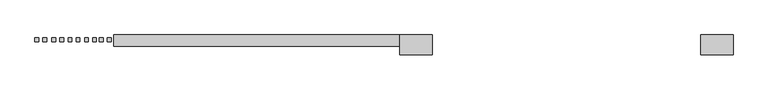
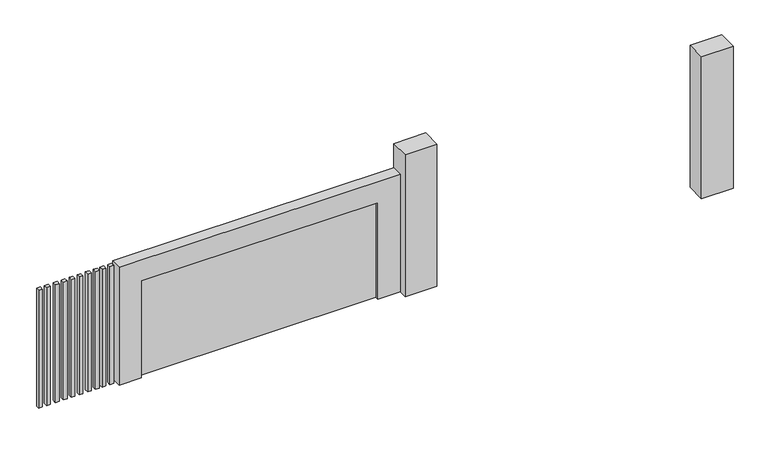
"""IFC4 building model written with IfcOpenShell, lengths in millimetres: proxy geometry."""

from ifc_helpers import new_model, si_unit, frame, origin, origin_with_axes, place, context, project, spatial, polyline, outline, extrude, source, transform, mapped, element, save


def generic_models_62b69d9f(model_context):
    return source(origin(), model_context, "Body", "SweptSolid", [
        extrude(outline(polyline([(-13668.6551496, -3549.697359), (-13617.8551496, -3549.697359), (-13617.8551496, -3600.497359), (-13668.6551496, -3600.497359), (-13668.6551496, -3549.697359)])), origin_with_axes(), (0.0, 0.0, 1.0), 1698.9467307),
        extrude(outline(polyline([(-13776.6051496, -3549.697359), (-13725.8051496, -3549.697359), (-13725.8051496, -3600.497359), (-13776.6051496, -3600.497359), (-13776.6051496, -3549.697359)])), origin_with_axes(), (0.0, 0.0, 1.0), 1698.9467307),
        extrude(outline(polyline([(-13440.0551496, -3549.697359), (-13389.2551496, -3549.697359), (-13389.2551496, -3600.497359), (-13440.0551496, -3600.497359), (-13440.0551496, -3549.697359)])), origin_with_axes(), (0.0, 0.0, 1.0), 1698.9467307),
        extrude(outline(polyline([(-13548.0051496, -3549.697359), (-13497.2051496, -3549.697359), (-13497.2051496, -3600.497359), (-13548.0051496, -3600.497359), (-13548.0051496, -3549.697359)])), origin_with_axes(), (0.0, 0.0, 1.0), 1698.9467307),
        extrude(outline(polyline([(-13224.1551496, -3549.697359), (-13173.3551496, -3549.697359), (-13173.3551496, -3600.497359), (-13224.1551496, -3600.497359), (-13224.1551496, -3549.697359)])), origin_with_axes(), (0.0, 0.0, 1.0), 1698.9467307),
        extrude(outline(polyline([(-13332.1051496, -3549.697359), (-13281.3051496, -3549.697359), (-13281.3051496, -3600.497359), (-13332.1051496, -3600.497359), (-13332.1051496, -3549.697359)])), origin_with_axes(), (0.0, 0.0, 1.0), 1698.9467307),
        extrude(outline(polyline([(-13001.9051496, -3549.697359), (-12951.1051496, -3549.697359), (-12951.1051496, -3600.497359), (-13001.9051496, -3600.497359), (-13001.9051496, -3549.697359)])), origin_with_axes(), (0.0, 0.0, 1.0), 1698.9467307),
        extrude(outline(polyline([(-13109.8551496, -3549.697359), (-13059.0551496, -3549.697359), (-13059.0551496, -3600.497359), (-13109.8551496, -3600.497359), (-13109.8551496, -3549.697359)])), origin_with_axes(), (0.0, 0.0, 1.0), 1698.9467307),
        extrude(outline(polyline([(-12805.0551496, -3549.697359), (-12754.2551496, -3549.697359), (-12754.2551496, -3600.497359), (-12805.0551496, -3600.497359), (-12805.0551496, -3549.697359)])), origin_with_axes(), (0.0, 0.0, 1.0), 1698.9467307),
        extrude(outline(polyline([(-12913.0051496, -3549.697359), (-12862.2051496, -3549.697359), (-12862.2051496, -3600.497359), (-12913.0051496, -3600.497359), (-12913.0051496, -3549.697359)])), origin_with_axes(), (0.0, 0.0, 1.0), 1698.9467307),
        extrude(outline(polyline([(-4410.3551496, -3511.597359), (-4410.3551496, -3778.297359), (-4843.5654887, -3778.297359), (-4843.5654887, -3511.597359), (-4410.3551496, -3511.597359)])), origin_with_axes(), (0.0, 0.0, 1.0), 2047.8276042),
        extrude(outline(polyline([(-8448.9551496, -3511.597359), (-8448.9551496, -3778.297359), (-8882.1654887, -3778.297359), (-8882.1654887, -3511.597359), (-8448.9551496, -3511.597359)])), origin_with_axes(), (0.0, 0.0, 1.0), 2047.8276042),
        extrude(outline(polyline([(-12411.3551496, -3613.197359), (-12411.3551496, -3511.597359), (-9186.9654887, -3511.597359), (-9186.9654887, -3613.197359), (-12411.3551496, -3613.197359)])), origin_with_axes(), (0.0, 0.0, 1.0), 1394.1467307),
        extrude(outline(polyline([(1698.9467307, -8882.1654887), (1698.9467307, -12716.1551496), (0.0, -12716.1551496), (0.0, -12411.3551496), (1394.1467307, -12411.3551496), (1394.1467307, -9186.9654887), (0.0, -9186.9654887), (0.0, -8882.1654887), (1698.9467307, -8882.1654887)])), frame((0.0, -3663.997359, 0.0), z_axis=(0.0, 1.0, 0.0), x_axis=(0.0, 0.0, 1.0)), (0.0, 0.0, 1.0), 152.4),
    ])


if __name__ == "__main__":
    model = new_model("IFC4")
    model_context = context("Model", 3, world=origin())
    ifc_project = project(units=[si_unit("LENGTHUNIT", "METRE", prefix="MILLI")], contexts=[model_context])
    site = spatial("IfcSite", under=ifc_project)
    building = spatial("IfcBuilding", under=site)
    placement = place(None, origin())
    generic_models_shape = generic_models_62b69d9f(model_context)
    element("IfcBuildingElementProxy", 1, Name="Generic Models", at=placement, inside=building, context=model_context, shape_type="MappedRepresentation", body=[
        mapped(generic_models_shape, transform((0.0, 0.0, 0.0), x_axis=(1.0, 0.0, 0.0), y_axis=(0.0, 1.0, 0.0), z_axis=(0.0, 0.0, 1.0))),
    ])
    save(model, "model.ifc")

# Revit data of these elements
# Element 1 (IfcBuildingElementProxy)
#   Materials on its faces: "Roofing, EPDM Membrane", "wall", "Gypsum Wall Board", "Door - Frame"
# Materials
#   "Roofing, EPDM Membrane": class "Generic", colour RGB 127 127 127, transparency 0, Description = "EPDM roof membrane", Cost = 0
#   "wall": class "Generic", colour RGB 120 120 120, transparency 0, Cost = 0
#   "Gypsum Wall Board": class "Generic", colour RGB 127 127 127, transparency 0, Description = "Gypsum Wall Board", Cost = 0
#   "Door - Frame": colour RGB 118 70 51, transparency 0, Cost = 0
